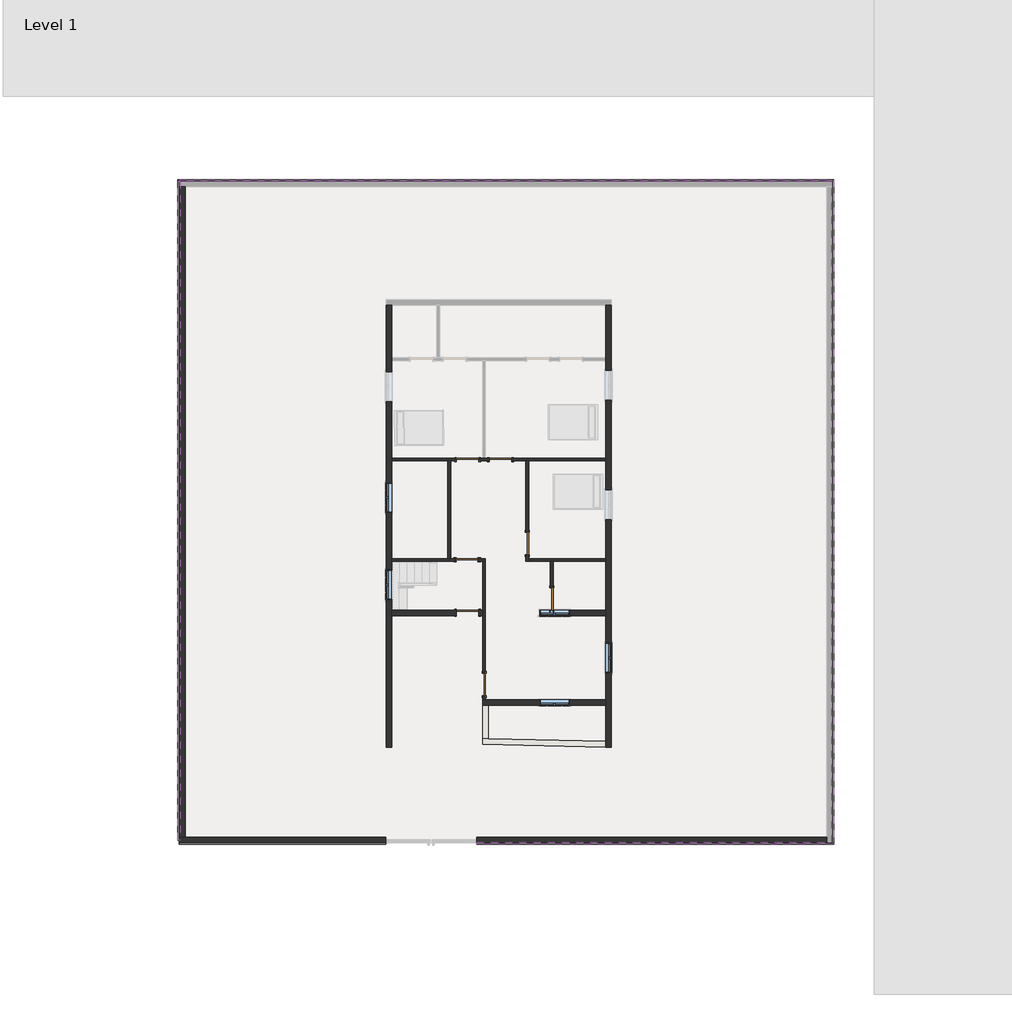
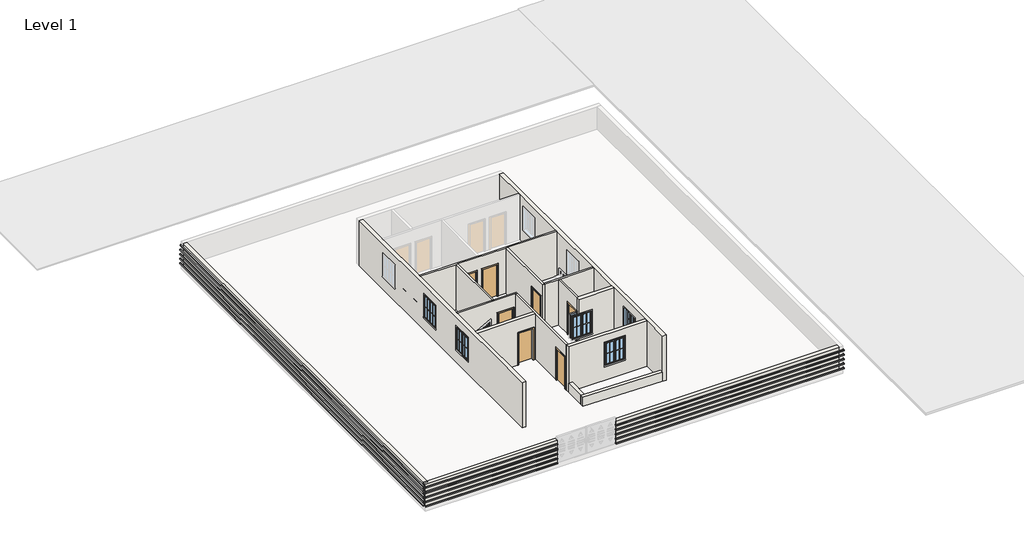
# One storey, part 1 of 3: 17 walls, 11 proxies, 8 doors, 5 windows.
"""IFC4 building model written with IfcOpenShell, lengths in millimetres."""

from ifc_helpers import new_model, si_unit, frame, origin, origin_with_axes, place, context, project, spatial, polyline, outline, extrude, faceted_brep, transform, mapped, element, save
from components import door_e5f9f3c4, door_305aa2a5, door_0ca8825f, window_8377141f

model = new_model("IFC4")

# Units and contexts
model_context = context("Model", 3, world=origin())
ifc_project = project(units=[si_unit("LENGTHUNIT", "METRE", prefix="MILLI")], contexts=[model_context])

# Site, building, storey
site = spatial("IfcSite", under=ifc_project)
building = spatial("IfcBuilding", under=site)
storey = spatial("IfcBuildingStorey", under=building, Name="Level 1", Elevation=0.0)

# Proxies
placement = place(None, origin())
element("IfcBuildingElementProxy", 1, Name="Reveal", ObjectType="Reveal", at=placement, inside=storey, context=model_context, shape_type="SweptSolid", body=[
    extrude(outline(polyline([(19370.729742, -8066.8365772), (19462.804742, -8158.9115772), (4956.229742, -8158.9115772), (4956.229742, -8066.8365772), (19370.729742, -8066.8365772)])), origin_with_axes(), (0.0, 0.0, 1.0), 67.7333333),
    extrude(outline(polyline([(19370.729742, 18755.5634228), (19462.804742, 18847.6384228), (19462.804742, -8158.9115772), (19370.729742, -8066.8365772), (19370.729742, 18755.5634228)])), origin_with_axes(), (0.0, 0.0, 1.0), 67.7333333),
    extrude(outline(polyline([(-7096.070258, 18755.5634228), (-7188.145258, 18847.6384228), (19462.804742, 18847.6384228), (19370.729742, 18755.5634228), (-7096.070258, 18755.5634228)])), origin_with_axes(), (0.0, 0.0, 1.0), 67.7333333),
])
element("IfcBuildingElementProxy", 2, Name="Reveal", ObjectType="Reveal", at=placement, inside=storey, context=model_context, shape_type="SweptSolid", body=[
    extrude(outline(polyline([(-7096.070258, -7977.9365772), (-7188.145258, -7977.9365772), (-7188.145258, 18847.6384228), (-7096.070258, 18755.5634228), (-7096.070258, -7977.9365772)])), origin_with_axes(), (0.0, 0.0, 1.0), 67.7333333),
    extrude(outline(polyline([(1259.3654616, -8066.8365772), (1259.3654616, -8158.9115772), (-7122.6345384, -8158.9115772), (-7122.6345384, -8066.8365772), (1259.3654616, -8066.8365772)])), origin_with_axes(), (0.0, 0.0, 1.0), 67.7333333),
])
element("IfcBuildingElementProxy", 3, Name="Reveal", ObjectType="Reveal", at=placement, inside=storey, context=model_context, shape_type="SweptSolid", body=[
    extrude(outline(polyline([(19370.729742, -8066.8365772), (19462.804742, -8158.9115772), (4956.229742, -8158.9115772), (4956.229742, -8066.8365772), (19370.729742, -8066.8365772)])), frame((0.0, 0.0, 304.8), z_axis=(0.0, 0.0, 1.0), x_axis=(1.0, 0.0, 0.0)), (0.0, 0.0, 1.0), 67.7333333),
    extrude(outline(polyline([(19370.729742, 18755.5634228), (19462.804742, 18847.6384228), (19462.804742, -8158.9115772), (19370.729742, -8066.8365772), (19370.729742, 18755.5634228)])), frame((0.0, 0.0, 304.8), z_axis=(0.0, 0.0, 1.0), x_axis=(1.0, 0.0, 0.0)), (0.0, 0.0, 1.0), 67.7333333),
    extrude(outline(polyline([(-7096.070258, 18755.5634228), (-7188.145258, 18847.6384228), (19462.804742, 18847.6384228), (19370.729742, 18755.5634228), (-7096.070258, 18755.5634228)])), frame((0.0, 0.0, 304.8), z_axis=(0.0, 0.0, 1.0), x_axis=(1.0, 0.0, 0.0)), (0.0, 0.0, 1.0), 67.7333333),
])
element("IfcBuildingElementProxy", 4, Name="Reveal", ObjectType="Reveal", at=placement, inside=storey, context=model_context, shape_type="SweptSolid", body=[
    extrude(outline(polyline([(19370.729742, -8066.8365772), (19462.804742, -8158.9115772), (4956.229742, -8158.9115772), (4956.229742, -8066.8365772), (19370.729742, -8066.8365772)])), frame((0.0, 0.0, 609.6), z_axis=(0.0, 0.0, 1.0), x_axis=(1.0, 0.0, 0.0)), (0.0, 0.0, 1.0), 67.7333333),
    extrude(outline(polyline([(19370.729742, 18755.5634228), (19462.804742, 18847.6384228), (19462.804742, -8158.9115772), (19370.729742, -8066.8365772), (19370.729742, 18755.5634228)])), frame((0.0, 0.0, 609.6), z_axis=(0.0, 0.0, 1.0), x_axis=(1.0, 0.0, 0.0)), (0.0, 0.0, 1.0), 67.7333333),
    extrude(outline(polyline([(-7096.070258, 18755.5634228), (-7188.145258, 18847.6384228), (19462.804742, 18847.6384228), (19370.729742, 18755.5634228), (-7096.070258, 18755.5634228)])), frame((0.0, 0.0, 609.6), z_axis=(0.0, 0.0, 1.0), x_axis=(1.0, 0.0, 0.0)), (0.0, 0.0, 1.0), 67.7333333),
])
element("IfcBuildingElementProxy", 5, Name="Reveal", ObjectType="Reveal", at=placement, inside=storey, context=model_context, shape_type="SweptSolid", body=[
    extrude(outline(polyline([(19370.729742, -8066.8365772), (19462.804742, -8158.9115772), (4956.229742, -8158.9115772), (4956.229742, -8066.8365772), (19370.729742, -8066.8365772)])), frame((0.0, 0.0, 914.4), z_axis=(0.0, 0.0, 1.0), x_axis=(1.0, 0.0, 0.0)), (0.0, 0.0, 1.0), 67.7333333),
    extrude(outline(polyline([(19370.729742, 18755.5634228), (19462.804742, 18847.6384228), (19462.804742, -8158.9115772), (19370.729742, -8066.8365772), (19370.729742, 18755.5634228)])), frame((0.0, 0.0, 914.4), z_axis=(0.0, 0.0, 1.0), x_axis=(1.0, 0.0, 0.0)), (0.0, 0.0, 1.0), 67.7333333),
    extrude(outline(polyline([(-7096.070258, 18755.5634228), (-7188.145258, 18847.6384228), (19462.804742, 18847.6384228), (19370.729742, 18755.5634228), (-7096.070258, 18755.5634228)])), frame((0.0, 0.0, 914.4), z_axis=(0.0, 0.0, 1.0), x_axis=(1.0, 0.0, 0.0)), (0.0, 0.0, 1.0), 67.7333333),
])
element("IfcBuildingElementProxy", 6, Name="Reveal", ObjectType="Reveal", at=placement, inside=storey, context=model_context, shape_type="SweptSolid", body=[
    extrude(outline(polyline([(19370.729742, -8066.8365772), (19462.804742, -8158.9115772), (4956.229742, -8158.9115772), (4956.229742, -8066.8365772), (19370.729742, -8066.8365772)])), frame((0.0, 0.0, 1219.2), z_axis=(0.0, 0.0, 1.0), x_axis=(1.0, 0.0, 0.0)), (0.0, 0.0, 1.0), 67.7333333),
    extrude(outline(polyline([(19370.729742, 18755.5634228), (19462.804742, 18847.6384228), (19462.804742, -8158.9115772), (19370.729742, -8066.8365772), (19370.729742, 18755.5634228)])), frame((0.0, 0.0, 1219.2), z_axis=(0.0, 0.0, 1.0), x_axis=(1.0, 0.0, 0.0)), (0.0, 0.0, 1.0), 67.7333333),
    extrude(outline(polyline([(-7121.470258, 18755.5634228), (-7121.470258, 18847.6384228), (19462.804742, 18847.6384228), (19370.729742, 18755.5634228), (-7121.470258, 18755.5634228)])), frame((0.0, 0.0, 1219.2), z_axis=(0.0, 0.0, 1.0), x_axis=(1.0, 0.0, 0.0)), (0.0, 0.0, 1.0), 67.7333333),
])
element("IfcBuildingElementProxy", 7, Name="Reveal", ObjectType="Reveal", at=placement, inside=storey, context=model_context, shape_type="SweptSolid", body=[
    extrude(outline(polyline([(-7096.070258, -7977.9365772), (-7188.145258, -7977.9365772), (-7188.145258, 18847.6384228), (-7096.070258, 18755.5634228), (-7096.070258, -7977.9365772)])), frame((0.0, 0.0, 304.8), z_axis=(0.0, 0.0, 1.0), x_axis=(1.0, 0.0, 0.0)), (0.0, 0.0, 1.0), 67.7333333),
    extrude(outline(polyline([(1259.3654616, -8066.8365772), (1259.3654616, -8158.9115772), (-7122.6345384, -8158.9115772), (-7122.6345384, -8066.8365772), (1259.3654616, -8066.8365772)])), frame((0.0, 0.0, 304.8), z_axis=(0.0, 0.0, 1.0), x_axis=(1.0, 0.0, 0.0)), (0.0, 0.0, 1.0), 67.7333333),
])
element("IfcBuildingElementProxy", 8, Name="Reveal", ObjectType="Reveal", at=placement, inside=storey, context=model_context, shape_type="SweptSolid", body=[
    extrude(outline(polyline([(-7096.070258, -7977.9365772), (-7188.145258, -7977.9365772), (-7188.145258, 18847.6384228), (-7096.070258, 18755.5634228), (-7096.070258, -7977.9365772)])), frame((0.0, 0.0, 609.6), z_axis=(0.0, 0.0, 1.0), x_axis=(1.0, 0.0, 0.0)), (0.0, 0.0, 1.0), 67.7333333),
    extrude(outline(polyline([(1259.3654616, -8066.8365772), (1259.3654616, -8158.9115772), (-7122.6345384, -8158.9115772), (-7122.6345384, -8066.8365772), (1259.3654616, -8066.8365772)])), frame((0.0, 0.0, 609.6), z_axis=(0.0, 0.0, 1.0), x_axis=(1.0, 0.0, 0.0)), (0.0, 0.0, 1.0), 67.7333333),
])
element("IfcBuildingElementProxy", 9, Name="Reveal", ObjectType="Reveal", at=placement, inside=storey, context=model_context, shape_type="SweptSolid", body=[
    extrude(outline(polyline([(-7096.070258, -7977.9365772), (-7188.145258, -7977.9365772), (-7188.145258, 18847.6384228), (-7096.070258, 18755.5634228), (-7096.070258, -7977.9365772)])), frame((0.0, 0.0, 914.4), z_axis=(0.0, 0.0, 1.0), x_axis=(1.0, 0.0, 0.0)), (0.0, 0.0, 1.0), 67.7333333),
    extrude(outline(polyline([(1259.3654616, -8066.8365772), (1259.3654616, -8158.9115772), (-7122.6345384, -8158.9115772), (-7122.6345384, -8066.8365772), (1259.3654616, -8066.8365772)])), frame((0.0, 0.0, 914.4), z_axis=(0.0, 0.0, 1.0), x_axis=(1.0, 0.0, 0.0)), (0.0, 0.0, 1.0), 67.7333333),
])
element("IfcBuildingElementProxy", 10, Name="Reveal", ObjectType="Reveal", at=placement, inside=storey, context=model_context, shape_type="SweptSolid", body=[
    extrude(outline(polyline([(-7096.070258, -7977.9365772), (-7188.145258, -7977.9365772), (-7188.145258, 18780.9634228), (-7096.070258, 18780.9634228), (-7096.070258, -7977.9365772)])), frame((0.0, 0.0, 965.2), z_axis=(0.0, 0.0, 1.0), x_axis=(1.0, 0.0, 0.0)), (0.0, 0.0, 1.0), 67.7333333),
    extrude(outline(polyline([(1259.3654616, -8066.8365772), (1259.3654616, -8158.9115772), (-7122.6345384, -8158.9115772), (-7122.6345384, -8066.8365772), (1259.3654616, -8066.8365772)])), frame((0.0, 0.0, 965.2), z_axis=(0.0, 0.0, 1.0), x_axis=(1.0, 0.0, 0.0)), (0.0, 0.0, 1.0), 67.7333333),
])
element("IfcBuildingElementProxy", 11, Name="Reveal", ObjectType="Reveal", at=placement, inside=storey, context=model_context, shape_type="SweptSolid", body=[
    extrude(outline(polyline([(-7096.070258, -7977.9365772), (-7188.145258, -7977.9365772), (-7188.145258, 18780.9634228), (-7096.070258, 18780.9634228), (-7096.070258, -7977.9365772)])), frame((0.0, 0.0, 1270.0), z_axis=(0.0, 0.0, 1.0), x_axis=(1.0, 0.0, 0.0)), (0.0, 0.0, 1.0), 67.7333333),
    extrude(outline(polyline([(1259.3654616, -8066.8365772), (1259.3654616, -8158.9115772), (-7122.6345384, -8158.9115772), (-7122.6345384, -8066.8365772), (1259.3654616, -8066.8365772)])), frame((0.0, 0.0, 1270.0), z_axis=(0.0, 0.0, 1.0), x_axis=(1.0, 0.0, 0.0)), (0.0, 0.0, 1.0), 67.7333333),
])

# Doors
door_shape = door_e5f9f3c4(model_context)
element("IfcDoor", 12, ObjectType="Single-Flush : 36\" x 84\"", at=placement, inside=storey, context=model_context, shape_type="MappedRepresentation", body=[
    mapped(door_shape, transform((4584.7, 7473.95, 0.0), x_axis=(1.0, 0.0, 0.0), y_axis=(0.0, 1.0, 0.0), z_axis=(0.0, 0.0, 1.0))),
])
element("IfcDoor", 13, ObjectType="Single-Flush : 36\" x 84\"", at=placement, inside=storey, context=model_context, shape_type="MappedRepresentation", body=[
    mapped(door_shape, transform((4546.6, 3397.25, 0.0), x_axis=(1.0, 0.0, 0.0), y_axis=(0.0, 1.0, 0.0), z_axis=(0.0, 0.0, 1.0))),
])
element("IfcDoor", 14, ObjectType="Single-Flush : 36\" x 84\"", at=placement, inside=storey, context=model_context, shape_type="MappedRepresentation", body=[
    mapped(door_shape, transform((4584.7, 3397.25, 0.0), x_axis=(1.0, 0.0, 0.0), y_axis=(0.0, 1.0, 0.0), z_axis=(0.0, 0.0, 1.0))),
])
element("IfcDoor", 15, ObjectType="Single-Flush : 36\" x 84\"", at=placement, inside=storey, context=model_context, shape_type="MappedRepresentation", body=[
    mapped(door_shape, transform((7004.05, 4064.0, 0.0), x_axis=(0.0, -1.0, 0.0), y_axis=(1.0, 0.0, 0.0), z_axis=(0.0, 0.0, 1.0))),
])
element("IfcDoor", 16, ObjectType="Single-Flush : 36\" x 84\"", at=placement, inside=storey, context=model_context, shape_type="MappedRepresentation", body=[
    mapped(door_shape, transform((5251.45, -1663.7, 0.0), x_axis=(0.0, -1.0, 0.0), y_axis=(1.0, 0.0, 0.0), z_axis=(0.0, 0.0, 1.0))),
])
door_2_shape = door_305aa2a5(model_context)
element("IfcDoor", 17, ObjectType="Single-Flush : 36\" x 84\"", at=placement, inside=storey, context=model_context, shape_type="MappedRepresentation", body=[
    mapped(door_2_shape, transform((5918.2, 7473.95, 0.0), x_axis=(-1.0, 0.0, 0.0), y_axis=(0.0, -1.0, 0.0), z_axis=(0.0, 0.0, 1.0))),
])
element("IfcDoor", 18, ObjectType="Single-Flush : 36\" x 84\"", at=placement, inside=storey, context=model_context, shape_type="MappedRepresentation", body=[
    mapped(door_2_shape, transform((7994.65, 1816.1, 0.0), x_axis=(0.0, 1.0, 0.0), y_axis=(-1.0, 0.0, 0.0), z_axis=(0.0, 0.0, 1.0))),
])
door_3_shape = door_0ca8825f(model_context)
element("IfcDoor", 19, ObjectType="Single-Flush : 36\" x 84\"", at=placement, inside=storey, context=model_context, shape_type="MappedRepresentation", body=[
    mapped(door_3_shape, transform((4584.7, 1244.6, 0.0), x_axis=(1.0, 0.0, 0.0), y_axis=(0.0, 1.0, 0.0), z_axis=(0.0, 0.0, 1.0))),
])

# Walls
element("IfcWall", 20, ObjectType="Generic - 5\"", at=placement, inside=storey, context=model_context, shape_type="Brep", body=[
    faceted_brep([(5041.9, 7416.8, 2133.6), (5041.9, 7416.8, 0.0), (5461.0, 7416.8, 0.0), (5461.0, 7416.8, 2133.6), (6375.4, 7416.8, 2133.6), (6375.4, 7416.8, 0.0), (6946.9, 7416.8, 0.0), (7061.2, 7416.8, 0.0), (10185.4, 7416.8, 0.0), (10185.4, 7416.8, 3048.0), (7061.2, 7416.8, 3048.0), (6946.9, 7416.8, 3048.0), (3898.9, 7416.8, 3048.0), (3784.6, 7416.8, 3048.0), (1498.6, 7416.8, 3048.0), (1498.6, 7416.8, 0.0), (3784.6, 7416.8, 0.0), (3898.9, 7416.8, 0.0), (4127.5, 7416.8, 0.0), (4127.5, 7416.8, 2133.6), (5461.0, 7531.1, 0.0), (5308.6, 7531.1, 0.0), (5194.3, 7531.1, 0.0), (5041.9, 7531.1, 0.0), (5041.9, 7531.1, 2133.6), (4127.5, 7531.1, 2133.6), (4127.5, 7531.1, 0.0), (1498.6, 7531.1, 0.0), (1498.6, 7531.1, 3048.0), (5194.3, 7531.1, 3048.0), (5308.6, 7531.1, 3048.0), (10185.4, 7531.1, 3048.0), (10185.4, 7531.1, 0.0), (6375.4, 7531.1, 0.0), (6375.4, 7531.1, 2133.6), (5461.0, 7531.1, 2133.6)], [[[0, 1, 2, 3, 4, 5, 6, 7, 8, 9, 10, 11, 12, 13, 14, 15, 16, 17, 18, 19]], [[20, 21, 22, 23, 24, 25, 26, 27, 28, 29, 30, 31, 32, 33, 34, 35]], [[33, 32, 8, 7, 6, 5]], [[2, 1, 23, 22, 21, 20]], [[18, 17, 16, 15, 27, 26]], [[14, 13, 12, 11, 10, 9, 31, 30, 29, 28]], [[9, 8, 32, 31]], [[15, 14, 28, 27]], [[3, 2, 20, 35]], [[4, 3, 35, 34]], [[5, 4, 34, 33]], [[24, 23, 1, 0]], [[25, 24, 0, 19]], [[26, 25, 19, 18]]]),
])
element("IfcWall", 21, ObjectType="Generic - 5\"", at=placement, inside=storey, context=model_context, shape_type="SweptSolid", body=[
    extrude(outline(polyline([(3784.6, 3454.4), (3784.6, 7416.8), (3898.9, 7416.8), (3898.9, 3454.4), (3784.6, 3454.4)])), origin_with_axes(), (0.0, 0.0, 1.0), 3048.0),
])
element("IfcWall", 22, ObjectType="Generic - 5\"", at=placement, inside=storey, context=model_context, shape_type="Brep", body=[
    faceted_brep([(5308.6, 3340.1, 3048.0), (5194.3, 3340.1, 3048.0), (1498.6, 3340.1, 3048.0), (1498.6, 3340.1, 0.0), (4089.4, 3340.1, 0.0), (4089.4, 3340.1, 2133.6), (5041.9, 3340.1, 2133.6), (5041.9, 3340.1, 0.0), (5194.3, 3340.1, 0.0), (5308.6, 3340.1, 0.0), (1498.6, 3454.4, 3048.0), (3784.6, 3454.4, 3048.0), (3898.9, 3454.4, 3048.0), (5308.6, 3454.4, 3048.0), (5308.6, 3454.4, 0.0), (5041.9, 3454.4, 0.0), (5041.9, 3454.4, 2133.6), (4089.4, 3454.4, 2133.6), (4089.4, 3454.4, 0.0), (3898.9, 3454.4, 0.0), (3784.6, 3454.4, 0.0), (1498.6, 3454.4, 0.0)], [[[0, 1, 2, 3, 4, 5, 6, 7, 8, 9]], [[10, 11, 12, 13, 14, 15, 16, 17, 18, 19, 20, 21]], [[3, 21, 20, 19, 18, 4]], [[14, 9, 8, 7, 15]], [[2, 1, 0, 13, 12, 11, 10]], [[3, 2, 10, 21]], [[0, 9, 14, 13]], [[5, 17, 16, 6]], [[18, 17, 5, 4]], [[6, 16, 15, 7]]]),
])
element("IfcWall", 23, ObjectType="Generic - 5\"", at=placement, inside=storey, context=model_context, shape_type="Brep", body=[
    faceted_brep([(5194.3, -2120.9, 2133.6), (5194.3, -2120.9, 0.0), (5194.3, -2286.0, 0.0), (5194.3, -2286.0, 3048.0), (5194.3, 1130.3, 3048.0), (5194.3, 1358.9, 3048.0), (5194.3, 3340.1, 3048.0), (5194.3, 3340.1, 0.0), (5194.3, 1358.9, 0.0), (5194.3, 1130.3, 0.0), (5194.3, -1206.5, 0.0), (5194.3, -1206.5, 2133.6), (5308.6, -2286.0, 0.0), (5308.6, -2120.9, 0.0), (5308.6, -2120.9, 2133.6), (5308.6, -1206.5, 2133.6), (5308.6, -1206.5, 0.0), (5308.6, 3340.1, 0.0), (5308.6, 3340.1, 3048.0), (5308.6, -2286.0, 3048.0)], [[[0, 1, 2, 3, 4, 5, 6, 7, 8, 9, 10, 11]], [[12, 13, 14, 15, 16, 17, 18, 19]], [[2, 1, 13, 12]], [[10, 9, 8, 7, 17, 16]], [[6, 5, 4, 3, 19, 18]], [[7, 6, 18, 17]], [[3, 2, 12, 19]], [[14, 13, 1, 0]], [[15, 14, 0, 11]], [[16, 15, 11, 10]]]),
])
element("IfcWall", 24, ObjectType="Generic - 5\"", at=placement, inside=storey, context=model_context, shape_type="Brep", body=[
    faceted_brep([(6946.9, 3606.8, 2133.6), (6946.9, 3606.8, 0.0), (6946.9, 3340.1, 0.0), (6946.9, 3340.1, 3048.0), (6946.9, 7416.8, 3048.0), (6946.9, 7416.8, 0.0), (6946.9, 4521.2, 0.0), (6946.9, 4521.2, 2133.6), (7061.2, 3340.1, 0.0), (7061.2, 3454.4, 0.0), (7061.2, 3606.8, 0.0), (7061.2, 3606.8, 2133.6), (7061.2, 4521.2, 2133.6), (7061.2, 4521.2, 0.0), (7061.2, 7416.8, 0.0), (7061.2, 7416.8, 3048.0), (7061.2, 3454.4, 3048.0), (7061.2, 3340.1, 3048.0)], [[[0, 1, 2, 3, 4, 5, 6, 7]], [[8, 9, 10, 11, 12, 13, 14, 15, 16, 17]], [[6, 5, 14, 13]], [[2, 1, 10, 9, 8]], [[4, 3, 17, 16, 15]], [[5, 4, 15, 14]], [[3, 2, 8, 17]], [[11, 10, 1, 0]], [[12, 11, 0, 7]], [[13, 12, 7, 6]]]),
])
element("IfcWall", 25, ObjectType="Generic - 5\"", at=placement, inside=storey, context=model_context, shape_type="SweptSolid", body=[
    extrude(outline(polyline([(1358.9, 3048.0), (3340.1, 3048.0), (3340.1, 0.0), (2273.3, 0.0), (2273.3, 2133.6), (1358.9, 2133.6), (1358.9, 3048.0)])), frame((7937.5, 0.0, 0.0), z_axis=(1.0, 0.0, 0.0), x_axis=(0.0, 1.0, 0.0)), (0.0, 0.0, 1.0), 114.3),
])
element("IfcWall", 26, ObjectType="Generic - 5\"", at=placement, inside=storey, context=model_context, shape_type="Brep", body=[
    faceted_brep([(7061.2, 3340.1, 0.0), (7937.5, 3340.1, 0.0), (8051.8, 3340.1, 0.0), (10185.4, 3340.1, 0.0), (10185.4, 3340.1, 3048.0), (8051.8, 3340.1, 3048.0), (7937.5, 3340.1, 3048.0), (7061.2, 3340.1, 3048.0), (7061.2, 3454.4, 0.0), (7061.2, 3454.4, 3048.0), (10185.4, 3454.4, 3048.0), (10185.4, 3454.4, 0.0)], [[[0, 1, 2, 3, 4, 5, 6, 7]], [[8, 9, 10, 11]], [[3, 2, 1, 0, 8, 11]], [[7, 6, 5, 4, 10, 9]], [[0, 7, 9, 8]], [[4, 3, 11, 10]]]),
])
element("IfcWall", 27, ObjectType="Generic - 8\"", at=placement, inside=storey, context=model_context, shape_type="Brep", body=[
    faceted_brep([(10185.4, 13741.4, 0.0), (10185.4, 11607.8, 0.0), (10185.4, 11493.5, 0.0), (10185.4, 7531.1, 0.0), (10185.4, 7416.8, 0.0), (10185.4, 3454.4, 0.0), (10185.4, 3340.1, 0.0), (10185.4, 1358.9, 0.0), (10185.4, 1130.3, 0.0), (10185.4, -2286.0, 0.0), (10185.4, -2514.6, 0.0), (10185.4, -3975.0400638, 0.0), (10185.4, -4203.7, 0.0), (10185.4, -4203.7, 609.6), (10185.4, -4203.7, 3048.0), (10185.4, -2514.6, 3048.0), (10185.4, -2286.0, 3048.0), (10185.4, 1130.3, 3048.0), (10185.4, 1358.9, 3048.0), (10185.4, 3340.1, 3048.0), (10185.4, 3454.4, 3048.0), (10185.4, 7416.8, 3048.0), (10185.4, 7531.1, 3048.0), (10185.4, 11493.5, 3048.0), (10185.4, 11607.8, 3048.0), (10185.4, 13741.4, 3048.0), (10185.4, 9874.25, 2438.4), (10185.4, 9874.25, 914.4), (10185.4, 11093.45, 914.4), (10185.4, 11093.45, 2438.4), (10185.4, 5035.55, 2438.4), (10185.4, 5035.55, 914.4), (10185.4, 6254.75, 914.4), (10185.4, 6254.75, 2438.4), (10185.4, -1187.45, 2438.4), (10185.4, -1187.45, 914.4), (10185.4, 31.75, 914.4), (10185.4, 31.75, 2438.4), (10414.0, 13741.4, 0.0), (10414.0, 13741.4, 3048.0), (10414.0, -4208.9351145, 3048.0), (10414.0, -4208.9351145, 0.0), (10414.0, 9874.25, 2438.4), (10414.0, 11093.45, 2438.4), (10414.0, 11093.45, 914.4), (10414.0, 9874.25, 914.4), (10414.0, 5035.55, 2438.4), (10414.0, 6254.75, 2438.4), (10414.0, 6254.75, 914.4), (10414.0, 5035.55, 914.4), (10414.0, -1187.45, 2438.4), (10414.0, 31.75, 2438.4), (10414.0, 31.75, 914.4), (10414.0, -1187.45, 914.4)], [[[0, 1, 2, 3, 4, 5, 6, 7, 8, 9, 10, 11, 12, 13, 14, 15, 16, 17, 18, 19, 20, 21, 22, 23, 24, 25], [26, 27, 28, 29], [30, 31, 32, 33], [34, 35, 36, 37]], [[38, 39, 40, 41], [42, 43, 44, 45], [46, 47, 48, 49], [50, 51, 52, 53]], [[12, 11, 10, 9, 8, 7, 6, 5, 4, 3, 2, 1, 0, 38, 41]], [[0, 25, 39, 38]], [[27, 26, 42, 45]], [[28, 27, 45, 44]], [[29, 28, 44, 43]], [[26, 29, 43, 42]], [[31, 30, 46, 49]], [[32, 31, 49, 48]], [[33, 32, 48, 47]], [[30, 33, 47, 46]], [[35, 34, 50, 53]], [[36, 35, 53, 52]], [[37, 36, 52, 51]], [[34, 37, 51, 50]], [[25, 24, 23, 22, 21, 20, 19, 18, 17, 16, 15, 14, 40, 39]], [[14, 13, 12, 41, 40]]]),
])
element("IfcWall", 28, ObjectType="Generic - 8\"", at=placement, inside=storey, context=model_context, shape_type="Brep", body=[
    faceted_brep([(1498.6, -4203.7, 0.0), (1498.6, 1130.3, 0.0), (1498.6, 1358.9, 0.0), (1498.6, 3340.1, 0.0), (1498.6, 3454.4, 0.0), (1498.6, 7416.8, 0.0), (1498.6, 7531.1, 0.0), (1498.6, 11493.5, 0.0), (1498.6, 11607.8, 0.0), (1498.6, 13741.4, 0.0), (1498.6, 13741.4, 3048.0), (1498.6, 11607.8, 3048.0), (1498.6, 11493.5, 3048.0), (1498.6, 7531.1, 3048.0), (1498.6, 7416.8, 3048.0), (1498.6, 3454.4, 3048.0), (1498.6, 3340.1, 3048.0), (1498.6, 1358.9, 3048.0), (1498.6, 1130.3, 3048.0), (1498.6, -4203.7, 3048.0), (1498.6, 6534.15, 2438.4), (1498.6, 6534.15, 914.4), (1498.6, 5314.95, 914.4), (1498.6, 5314.95, 2438.4), (1498.6, 11042.65, 2438.4), (1498.6, 11042.65, 914.4), (1498.6, 9823.45, 914.4), (1498.6, 9823.45, 2438.4), (1498.6, 2990.85, 2438.4), (1498.6, 2990.85, 914.4), (1498.6, 1771.65, 914.4), (1498.6, 1771.65, 2438.4), (1270.0, -4203.7, 0.0), (1270.0, -4203.7, 3048.0), (1270.0, 13741.4, 3048.0), (1270.0, 13741.4, 0.0), (1270.0, 6534.15, 2438.4), (1270.0, 5314.95, 2438.4), (1270.0, 5314.95, 914.4), (1270.0, 6534.15, 914.4), (1270.0, 11042.65, 2438.4), (1270.0, 9823.45, 2438.4), (1270.0, 9823.45, 914.4), (1270.0, 11042.65, 914.4), (1270.0, 2990.85, 2438.4), (1270.0, 1771.65, 2438.4), (1270.0, 1771.65, 914.4), (1270.0, 2990.85, 914.4)], [[[0, 1, 2, 3, 4, 5, 6, 7, 8, 9, 10, 11, 12, 13, 14, 15, 16, 17, 18, 19], [20, 21, 22, 23], [24, 25, 26, 27], [28, 29, 30, 31]], [[32, 33, 34, 35], [36, 37, 38, 39], [40, 41, 42, 43], [44, 45, 46, 47]], [[9, 8, 7, 6, 5, 4, 3, 2, 1, 0, 32, 35]], [[0, 19, 33, 32]], [[10, 9, 35, 34]], [[21, 20, 36, 39]], [[22, 21, 39, 38]], [[23, 22, 38, 37]], [[20, 23, 37, 36]], [[25, 24, 40, 43]], [[26, 25, 43, 42]], [[27, 26, 42, 41]], [[24, 27, 41, 40]], [[29, 28, 44, 47]], [[30, 29, 47, 46]], [[31, 30, 46, 45]], [[28, 31, 45, 44]], [[19, 18, 17, 16, 15, 14, 13, 12, 11, 10, 34, 33]]]),
])
element("IfcWall", 29, ObjectType="Generic - 8\"", at=placement, inside=storey, context=model_context, shape_type="SweptSolid", body=[
    extrude(outline(polyline([(2133.6, 5041.9), (0.0, 5041.9), (0.0, 5194.3), (3048.0, 5194.3), (3048.0, 1498.6), (0.0, 1498.6), (0.0, 4127.5), (2133.6, 4127.5), (2133.6, 5041.9)])), frame((0.0, 1130.3, 0.0), z_axis=(0.0, 1.0, 0.0), x_axis=(0.0, 0.0, 1.0)), (0.0, 0.0, 1.0), 228.6),
])
element("IfcWall", 30, ObjectType="Generic - 8\"", at=placement, inside=storey, context=model_context, shape_type="Brep", body=[
    faceted_brep([(5194.3, -2514.6, 3048.0), (5194.3, -2514.6, 609.6), (5194.3, -2514.6, 0.0), (5422.9, -2514.6, 0.0), (10185.4, -2514.6, 0.0), (10185.4, -2514.6, 3048.0), (7505.7, -2514.6, 2519.22095), (8724.9, -2514.6, 2519.22095), (8724.9, -2514.6, 995.22095), (7505.7, -2514.6, 995.22095), (5194.3, -2286.0, 0.0), (5194.3, -2286.0, 3048.0), (5308.6, -2286.0, 3048.0), (10185.4, -2286.0, 3048.0), (10185.4, -2286.0, 0.0), (5308.6, -2286.0, 0.0), (7505.7, -2286.0, 2519.22095), (7505.7, -2286.0, 995.22095), (8724.9, -2286.0, 995.22095), (8724.9, -2286.0, 2519.22095)], [[[0, 1, 2, 3, 4, 5], [6, 7, 8, 9]], [[10, 11, 12, 13, 14, 15], [16, 17, 18, 19]], [[4, 3, 2, 10, 15, 14]], [[5, 4, 14, 13]], [[0, 5, 13, 12, 11]], [[0, 11, 10, 2, 1]], [[17, 16, 6, 9]], [[18, 17, 9, 8]], [[19, 18, 8, 7]], [[16, 19, 7, 6]]]),
])
element("IfcWall", 31, ObjectType="Generic - 8\"", at=placement, inside=storey, context=model_context, shape_type="Brep", body=[
    faceted_brep([(7937.5, 1130.3, 0.0), (10185.4, 1130.3, 0.0), (10185.4, 1130.3, 3048.0), (7937.5, 1130.3, 3048.0), (7937.5, 1130.3, 2046.4565505), (8731.25, 1130.3, 2046.4565505), (8731.25, 1130.3, 522.4565505), (7937.5, 1130.3, 522.4565505), (10185.4, 1358.9, 0.0), (7937.5, 1358.9, 0.0), (7937.5, 1358.9, 522.4565505), (8731.25, 1358.9, 522.4565505), (8731.25, 1358.9, 2046.4565505), (7937.5, 1358.9, 2046.4565505), (7937.5, 1358.9, 2133.6), (7937.5, 1358.9, 3048.0), (8051.8, 1358.9, 3048.0), (10185.4, 1358.9, 3048.0)], [[[0, 1, 2, 3, 4, 5, 6, 7]], [[8, 9, 10, 11, 12, 13, 14, 15, 16, 17]], [[1, 0, 9, 8]], [[9, 0, 7, 10]], [[3, 15, 14, 13, 4]], [[2, 1, 8, 17]], [[3, 2, 17, 16, 15]], [[6, 11, 10, 7]], [[11, 6, 5, 12]], [[12, 5, 4, 13]]]),
])
element("IfcWall", 32, ObjectType="Generic - 8\"", at=placement, inside=storey, context=model_context, shape_type="SweptSolid", body=[
    extrude(outline(polyline([(-7863.6365772, 1524.0), (-7863.6365772, 0.0), (-8066.8365772, 0.0), (-8066.8365772, 67.7333333), (-8092.2365772, 67.7333333), (-8092.2365772, 304.8), (-8066.8365772, 304.8), (-8066.8365772, 372.5333333), (-8092.2365772, 372.5333333), (-8092.2365772, 609.6), (-8066.8365772, 609.6), (-8066.8365772, 677.3333333), (-8092.2365772, 677.3333333), (-8092.2365772, 914.4), (-8066.8365772, 914.4), (-8066.8365772, 982.1333333), (-8092.2365772, 982.1333333), (-8092.2365772, 1219.2), (-8066.8365772, 1219.2), (-8066.8365772, 1286.9333333), (-8092.2365772, 1286.9333333), (-8092.2365772, 1524.0), (-7863.6365772, 1524.0)])), frame((4956.229742, 0.0, 0.0), z_axis=(1.0, 0.0, 0.0), x_axis=(0.0, 1.0, 0.0)), (0.0, 0.0, 1.0), 14211.3),
])
element("IfcWall", 33, ObjectType="Generic - 8\"", at=placement, inside=storey, context=model_context, shape_type="SweptSolid", body=[
    extrude(outline(polyline([(0.0, -6892.870258), (1524.0, -6892.870258), (1524.0, -7121.470258), (1337.7333333, -7121.470258), (1337.7333333, -7096.070258), (1270.0, -7096.070258), (1270.0, -7121.470258), (1032.9333333, -7121.470258), (1032.9333333, -7096.070258), (914.4, -7096.070258), (914.4, -7121.470258), (677.3333333, -7121.470258), (677.3333333, -7096.070258), (609.6, -7096.070258), (609.6, -7121.470258), (372.5333333, -7121.470258), (372.5333333, -7096.070258), (304.8, -7096.070258), (304.8, -7121.470258), (67.7333333, -7121.470258), (67.7333333, -7096.070258), (0.0, -7096.070258), (0.0, -6892.870258)])), frame((0.0, -7977.9365772, 0.0), z_axis=(0.0, 1.0, 0.0), x_axis=(0.0, 0.0, 1.0)), (0.0, 0.0, 1.0), 26530.3),
])
element("IfcWall", 34, ObjectType="Generic - 8\"", at=placement, inside=storey, context=model_context, shape_type="Brep", body=[
    faceted_brep([(10185.4, -3975.0400638, 0.0), (5422.9, -3865.9751783, 0.0), (5194.3, -3860.7400638, 0.0), (5194.3, -3860.7400638, 609.6), (5422.9, -3865.9751783, 609.6), (10185.4, -3975.0400638, 609.6), (10185.4, -4203.7, 0.0), (10185.4, -4203.7, 609.6), (5194.3, -4089.4, 609.6), (5194.3, -4089.4, 0.0)], [[[0, 1, 2, 3, 4, 5]], [[6, 7, 8, 9]], [[2, 1, 0, 6, 9]], [[5, 4, 3, 8, 7]], [[0, 5, 7, 6]], [[3, 2, 9, 8]]]),
])
element("IfcWall", 35, ObjectType="Generic - 8\"", at=placement, inside=storey, context=model_context, shape_type="SweptSolid", body=[
    extrude(outline(polyline([(5422.9, -2514.6), (5422.9, -3865.9751783), (5194.3, -3860.7400638), (5194.3, -2514.6), (5422.9, -2514.6)])), origin_with_axes(), (0.0, 0.0, 1.0), 609.6),
])
element("IfcWall", 36, ObjectType="Generic - 8\"", at=placement, inside=storey, context=model_context, shape_type="SweptSolid", body=[
    extrude(outline(polyline([(-7863.6365772, 1524.0), (-7863.6365772, 0.0), (-8066.8365772, 0.0), (-8066.8365772, 67.7333333), (-8092.2365772, 67.7333333), (-8092.2365772, 304.8), (-8066.8365772, 304.8), (-8066.8365772, 372.5333333), (-8092.2365772, 372.5333333), (-8092.2365772, 609.6), (-8066.8365772, 609.6), (-8066.8365772, 677.3333333), (-8092.2365772, 677.3333333), (-8092.2365772, 914.4), (-8066.8365772, 914.4), (-8066.8365772, 1032.9333333), (-8092.2365772, 1032.9333333), (-8092.2365772, 1270.0), (-8066.8365772, 1270.0), (-8066.8365772, 1337.7333333), (-8092.2365772, 1337.7333333), (-8092.2365772, 1524.0), (-7863.6365772, 1524.0)])), frame((-7122.6345384, 0.0, 0.0), z_axis=(1.0, 0.0, 0.0), x_axis=(0.0, 1.0, 0.0)), (0.0, 0.0, 1.0), 8382.0),
])

# Windows
window_shape = window_8377141f(model_context)
element("IfcWindow", 37, ObjectType="Window-Casement-Double : 48\" x 60\"", at=placement, inside=storey, context=model_context, shape_type="MappedRepresentation", body=[
    mapped(window_shape, transform((1384.3, 5924.55, 0.0), x_axis=(0.0, 1.0, 0.0), y_axis=(-1.0, 0.0, 0.0), z_axis=(0.0, 0.0, 1.0))),
])
element("IfcWindow", 38, ObjectType="Window-Casement-Double : 48\" x 60\"", at=placement, inside=storey, context=model_context, shape_type="MappedRepresentation", body=[
    mapped(window_shape, transform((10299.7, -577.85, 0.0), x_axis=(0.0, -1.0, 0.0), y_axis=(1.0, 0.0, 0.0), z_axis=(0.0, 0.0, 1.0))),
])
element("IfcWindow", 39, ObjectType="Window-Casement-Double : 48\" x 60\"", at=placement, inside=storey, context=model_context, shape_type="MappedRepresentation", body=[
    mapped(window_shape, transform((1384.3, 2381.25, 0.0), x_axis=(0.0, 1.0, 0.0), y_axis=(-1.0, 0.0, 0.0), z_axis=(0.0, 0.0, 1.0))),
])
element("IfcWindow", 40, ObjectType="Window-Casement-Double : 48\" x 60\"", at=placement, inside=storey, context=model_context, shape_type="MappedRepresentation", body=[
    mapped(window_shape, transform((8121.65, 1244.6, -391.9434495), x_axis=(-1.0, 0.0, 0.0), y_axis=(0.0, -1.0, 0.0), z_axis=(0.0, 0.0, 1.0))),
])
element("IfcWindow", 41, ObjectType="Window-Casement-Double : 48\" x 60\"", at=placement, inside=storey, context=model_context, shape_type="MappedRepresentation", body=[
    mapped(window_shape, transform((8115.3, -2400.3, 80.82095), x_axis=(-1.0, 0.0, 0.0), y_axis=(0.0, -1.0, 0.0), z_axis=(0.0, 0.0, 1.0))),
])

save(model, "model.ifc")

# Revit data of these elements
# Type "Single-Flush : 36\" x 84\""
#   Type Mark = "1"
#   Construction Type Id = "MDOOR"
#   Assembly Code = "C1020"
#   Analytic Construction = "Metal"
#   Thickness = 0' - 2"
#   Heat Transfer Coefficient (U) = 0.651978 BTU/(h·ft²·°F)
#   Height = 7' - 0"
#   Trim Projection Ext = 0' - 1"
#   Trim Projection Int = 0' - 1"
#   Trim Width = 0' - 3"
#   Width = 3' - 0"
#   Define Thermal Properties by = 1
#   Define Thermal Properties by = 1
#   Door Material = Door - Panel
#   Frame Material = Door - Frame
#   Visual Light Transmittance = 0
#   Solar Heat Gain Coefficient = 0
#   Function = (empty or 0)
#   Wall Closure = (empty or 0)
# Type "Generic - 5\""
#   Assembly Code = "B2010"
#   Layers, outside or top first: 0' - 4 1/2" no material (function 1)
# Type "Generic - 8\""
#   Assembly Code = "B2010"
# Type "Window-Casement-Double : 48\" x 60\""
#   Type Mark = "17"
#   Fire Rating = "0.5h"
#   Assembly Code = "B2020100"
#   Analytic Construction = "Double glazing - domestic"
#   Frame Extension [instance default] = 0' - 0 1/4"
#   Window Inset [instance default] = 0' - 0"
#   Wall Thickness [instance default] = 0' - 6"
#   Interior Wall Closure [instance default] = 0' - 2 1/4"
#   Half Width = 2' - 0"
#   Visual Light Transmittance = 0.81
#   Thermal Resistance (R) = 1.8146 (h·ft²·°F)/BTU
#   Solar Heat Gain Coefficient = 0.76
#   Rough Width = 4' - 0 1/2"
#   Rough Height = 5' - 0 1/2"
#   Height = 5' - 0"
#   Heat Transfer Coefficient (U) = 0.5511 BTU/(h·ft²·°F)
#   Exterior Wall Closure [instance default] = 0' - 1 1/4"
#   Extension Jamb [instance default] = 0' - 2 1/4"
#   Default Sill Height = 3' - 0"
#   Width = 4' - 0"
#   Define Thermal Properties by = 0
#   Muntin Visibility = yes
#   Interior Trim Visibility [instance default] = yes
#   Exterior Trim Visibility [instance default] = yes
#   Extension Jamb Visibility [instance default] = yes
#   Interior Trim Material = Wood - Stained
#   Muntin Pattern = Muntin Pattern_2x2 : Muntin Pattern_2x2
#   Interior Trim = Trim-Window-Interior-Flat : Picture Frame
#   Interior Frame Material = Wood - Stained
#   Glass Panel Material = Glass
#   Exterior Trim Material = Clad - White
#   Exterior Trim = Trim-Window-Exterior-Flat : with Sill
#   Exterior Frame Material = Clad - White
#   Wall Closure = (empty or 0)
# Elements 12, 13, 14, 15, 16, 17, 18, 19 (IfcDoor, "Single-Flush : 36\" x 84\"")
#   Phase Created = New Construction
#   Materials on its faces: "Door - Frame", "Door - Panel"
# Elements 20, 21, 22, 24, 25, 26 (IfcWall, "Generic - 5\"")
#   Top Offset = 0' - 0"
#   Base Offset = 0' - 0"
#   wall height = 10' - 0"
#   Phase Created = New Construction
#   Base Constraint = Level 1
#   Top Constraint = Level 2
#   Materials on its faces: "Default Wall"
# Element 23 (IfcWall, "Generic - 5\"")
#   Top Offset = 0' - 0"
#   Base Offset = 0' - 0"
#   wall height = 10' - 0"
#   Phase Created = New Construction
#   Base Constraint = Level 1
#   Top Constraint = Level 2
#   Materials on its faces: "Default Wall", "Parking Stripe"
# Elements 27, 28, 29 (IfcWall, "Generic - 8\"")
#   Top Offset = 0' - 0"
#   Base Offset = 0' - 0"
#   Unconnected Height = 10' - 0"
#   wall height = 10' - 0"
#   Phase Created = New Construction
#   Base Constraint = Level 1
#   Materials on its faces: "Parking Stripe"
# Element 30 (IfcWall, "Generic - 8\"")
#   Top Offset = 0' - 0"
#   Base Offset = 0' - 0"
#   Unconnected Height = 10' - 0"
#   wall height = 10' - 0"
#   Phase Created = New Construction
#   Base Constraint = Level 1
#   Materials on its faces: "Parking Stripe", "Door - Panel"
# Element 31 (IfcWall, "Generic - 8\"")
#   Top Offset = 0' - 0"
#   Base Offset = 0' - 0"
#   Unconnected Height = 10' - 0"
#   wall height = 10' - 0"
#   Phase Created = New Construction
#   Base Constraint = Level 1
#   Materials on its faces: "Default Wall"
# Elements 32, 33, 36 (IfcWall, "Generic - 8\"")
#   Top Offset = 0' - 0"
#   Base Offset = 0' - 0"
#   Unconnected Height = 5' - 0"
#   wall height = 5' - 0"
#   Phase Created = New Construction
#   Base Constraint = Level 1
#   Materials on its faces: "Clad - White"
# Elements 34, 35 (IfcWall, "Generic - 8\"")
#   Top Offset = 0' - 0"
#   Base Offset = 0' - 0"
#   Unconnected Height = 2' - 0"
#   wall height = 2' - 0"
#   Phase Created = New Construction
#   Base Constraint = Level 1
#   Materials on its faces: "Door - Panel"
# Element 37 (IfcWindow, "Window-Casement-Double : 48\" x 60\"")
#   Mark = "1"
#   Window Inset = 0' - 0"
#   Interior Wall Closure = 0' - 2 1/4"
#   Frame Extension = 0' - 0 1/4"
#   Exterior Wall Closure = 0' - 1 1/4"
#   Interior Trim Visibility = yes
#   Exterior Trim Visibility = yes
#   Phase Created = New Construction
#   Materials on its faces: "Wood - Stained", "Glass", "Clad - White"
# Element 38 (IfcWindow, "Window-Casement-Double : 48\" x 60\"")
#   Mark = "5"
#   Window Inset = 0' - 0"
#   Interior Wall Closure = 0' - 2 1/4"
#   Frame Extension = 0' - 0 1/4"
#   Exterior Wall Closure = 0' - 1 1/4"
#   Interior Trim Visibility = yes
#   Exterior Trim Visibility = yes
#   Phase Created = New Construction
#   Materials on its faces: "Wood - Stained", "Glass", "Clad - White"
# Element 39 (IfcWindow, "Window-Casement-Double : 48\" x 60\"")
#   Mark = "7"
#   Window Inset = 0' - 0"
#   Interior Wall Closure = 0' - 2 1/4"
#   Frame Extension = 0' - 0 1/4"
#   Exterior Wall Closure = 0' - 1 1/4"
#   Interior Trim Visibility = yes
#   Exterior Trim Visibility = yes
#   Phase Created = New Construction
#   Materials on its faces: "Wood - Stained", "Glass", "Clad - White"
# Element 40 (IfcWindow, "Window-Casement-Double : 48\" x 60\"")
#   Mark = "32"
#   Window Inset = 0' - 0"
#   Interior Wall Closure = 0' - 2 1/4"
#   Frame Extension = 0' - 0 1/4"
#   Exterior Wall Closure = 0' - 1 1/4"
#   Interior Trim Visibility = yes
#   Exterior Trim Visibility = yes
#   Phase Created = New Construction
#   Materials on its faces: "Wood - Stained", "Glass", "Clad - White"
# Element 41 (IfcWindow, "Window-Casement-Double : 48\" x 60\"")
#   Mark = "33"
#   Window Inset = 0' - 0"
#   Interior Wall Closure = 0' - 2 1/4"
#   Frame Extension = 0' - 0 1/4"
#   Exterior Wall Closure = 0' - 1 1/4"
#   Interior Trim Visibility = yes
#   Exterior Trim Visibility = yes
#   Phase Created = New Construction
#   Materials on its faces: "Wood - Stained", "Glass", "Clad - White"
# Materials
#   "Door - Panel": class "Wood", colour RGB 210 159 95, transparency 0, Cost = 0
#   "Door - Frame": colour RGB 118 70 51, transparency 0, Cost = 0
#   "Wood - Stained": class "Wood", colour RGB 224 178 126, transparency 0, Cost = 0
#   "Glass": class "Glass", colour RGB 0 128 192, transparency 0.75, Description = "Soda Lime Glass", Cost = 0
#   "Clad - White": class "Wood", colour RGB 242 242 238, transparency 0, Cost = 0
#   "Default Wall": colour RGB 128 128 128, transparency 0, Cost = 0
#   "Parking Stripe": class "Paint", colour RGB 250 250 91, transparency 0, Cost = 0
